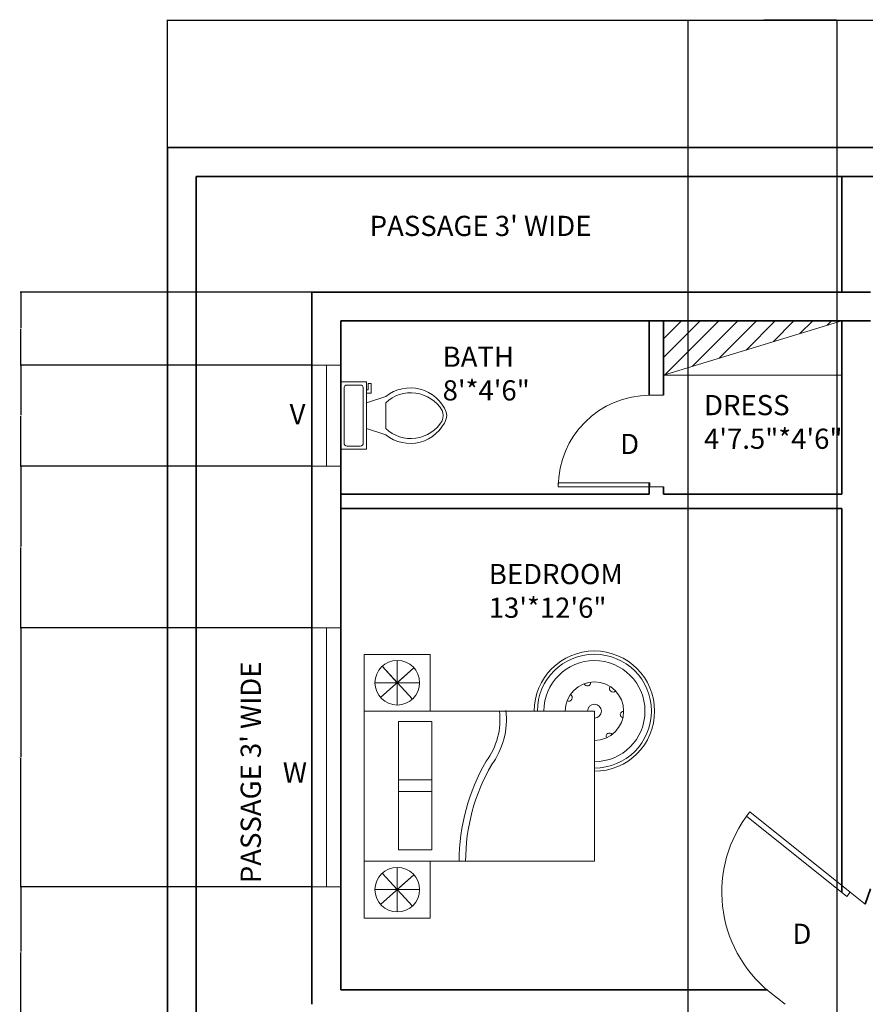
# Model space of a CAD drawing. Units: inches. Extents: x 2284 to 2815, y 1123 to 1948.
# Tile 5 of 6: x 2285 to 2548, y 1641 to 1948. Entities that reach past the tile are written whole.
import ezdxf

# ---------------------------------------------------------------- set-up
doc = ezdxf.new("R2010")
doc.units = ezdxf.units.IN
for name, color, linetype, lineweight in [('A-ANNO-DIMS', 2, 'Continuous', 18), ('A-AREA-IDEN', 30, 'Continuous', 18), ('A-CASE-PATT', 217, 'Continuous', 13), ('A-FLOR-CASE', 8, 'Continuous', 18), ('A-FLOR-FIXT', 9, 'Continuous', 18), ('A-WALL-PATT', 140, 'Continuous', 13), ('C-SITE-WALL', 7, 'Continuous', 35), ('DOOR', 190, 'Continuous', 18), ('FUR', 10, 'Continuous', 18), ('TEXT', 30, 'Continuous', 18), ('WALL', 7, 'Continuous', 35), ('WIND', 210, 'Continuous', 18)]:
    doc.layers.add(name, color=color, linetype=linetype, lineweight=lineweight)
doc.styles.get("Standard").update_dxf_attribs({"font": 'arial.ttf'})
doc.dimstyles.get("Standard").update_dxf_attribs({"dimtxt": 0.18, "dimasz": 0.18, "dimexe": 0.18, "dimexo": 0.0625, "dimgap": 0.09, "dimtad": 0, "dimtih": 1, "dimtoh": 1, "dimdec": 4, "dimzin": 0, "dimdsep": 46, "dimtxsty": 'Standard', "dimcen": 0.09, "dimadec": 0, "dimazin": 0, "dimtfac": 1, "dimtdec": 4, "dimtofl": 0, "dimtmove": 0, "dimatfit": 3, "dimfxl": 1, "dimtolj": 1, "dimtzin": 0, "dimarcsym": 0})

# ---------------------------------------------------------------- blocks, each defined once
blk = doc.blocks.new('*U2')
for p, q in [((0, 0), (0, -6)), ((40, 0), (40, -6))]:
    blk.add_line(p, q)
blk.add_lwpolyline([(0, 0), (0, 40), (1.75, 40), (1.75, 0)], close=True)
blk.add_arc((0, 0), 40, 0, 90)
blk = doc.blocks.new('*U4')
for p, q in [((9.5, -6), (9.5, -2)), ((-10, -8.5), (-8, -8.5)), ((-10, -9.5), (-10, -8.5)), ((-8, -8.5), (-8, -8)), ((-7, -8), (-7, -9.5)), ((-4, -8), (-6, -14)), ((4, -8), (6, -14)), ((-7, -9.5), (-10, -9.5)), ((4, -14), (-4, -14))]:
    blk.add_line(p, q)
blk.add_lwpolyline([(10.5, -8), (10.5, 0), (-10.5, 0), (-10.5, -8)], close=True)
for points in [[(-9.5, -2), (-9.5, -6)], [(8.5, -1), (-8.5, -1)], [(-8.5, -7), (8.5, -7)]]:
    blk.add_lwpolyline(points)
for centre, radius, start, end in [((-8.62, -1.88), 0.884, 81.8699, 188.1301), ((8.62, -1.88), 0.884, 351.8699, 98.1301), ((-8.62, -6.12), 0.884, 171.8699, 278.1301), ((8.62, -6.12), 0.884, 261.8699, 8.1301), ((3.52, -21.58), 12.17, 141.4691, 247.9714), ((4.2, -21.82), 11.33, 136.3677, 238.9468), ((-3.52, -21.58), 12.17, 292.0284, 38.5307), ((-4.2, -21.82), 11.33, 301.053, 43.6321), ((0, -27.88), 4, 245.7318, 294.2682), ((0, -29), 4, 254.8605, 285.1395)]:
    blk.add_arc(centre, radius, start, end)
blk = doc.blocks.new('BED-DOUBLE-WITH-RUG')
for points in [[(0, 0), (71.68, 0), (71.68, 46.8), (0, 46.8)], [(10.67, 21.75), (21.03, 21.75), (21.03, 43.61), (10.67, 43.61)], [(10.67, 3.58), (21.03, 3.58), (21.03, 25.43), (10.67, 25.43)]]:
    blk.add_lwpolyline(points, close=True)
for centre, radius, start, end in [((71.68, 46.8), 18.75, 270, 180), ((71.68, 46.8), 17.75, 270, 180), ((71.68, 46.8), 15.75, 270, 180), ((71.68, 46.8), 9.1, 270, 180), ((69.48, 55.63), 1, 197.1257, 10.8048), ((77.45, 53.83), 1.1, 144.137, 317.2027), ((63.62, 51.01), 1.12, 245.9164, 58.891), ((20.54, 44.16), 21.72, 323.3068, 6.9612), ((20.54, 44.16), 23.72, 323.3068, 6.9612), ((71.68, 46.8), 2.16, 270, 180), ((80.72, 45.75), 0.986, 86.4879, 260.2794), ((76.34, 38.98), 1, 33.9622, 207.6652), ((91.6, 0), 62.04, 149.8305, 180), ((91.6, 0), 60.04, 149.8305, 180)]:
    blk.add_arc(centre, radius, start, end)
blk = doc.blocks.new('NIGHTSTAND-LAMP')
for p, q in [((10.28, 1.89), (10.28, 15.8)), ((15.48, 13.46), (5.08, 4.23)), ((10.28, 8.85), (5.59, 13.98)), ((5.59, 13.98), (14.97, 3.71)), ((10.28, 8.85), (15.48, 13.46)), ((3.33, 8.85), (17.23, 8.85))]:
    blk.add_line(p, q)
blk.add_lwpolyline([(0, 0), (20.56, 0), (20.56, 17.69), (0, 17.69)], close=True)
blk.add_circle((10.28, 8.85), 6.95)
blk = doc.blocks.new('*D20')
at = {"layer": 'A-ANNO-DIMS', "color": 0, "lineweight": -2, "transparency": 16777216}
for p, q in [((2330.55, 1908.47), (2330.55, 1948.28)), ((2330.73, 1948.1), (2552.26, 1948.1)), ((2774.37, 1948.1), (2552.85, 1948.1)), ((2774.55, 1908.47), (2774.55, 1948.28))]:
    blk.add_line(p, q, dxfattribs=at)
at = {"layer": 'A-ANNO-DIMS', "color": 0, "transparency": 16777216}
for points in [[(2330.73, 1948.13), (2330.73, 1948.07), (2330.55, 1948.1)], [(2774.37, 1948.13), (2774.37, 1948.07), (2774.55, 1948.1)]]:
    blk.add_solid(points, dxfattribs=at)
at = {"layer": 'Defpoints', "color": 0, "transparency": 16777216}
for p in [(2774.55, 1948.1), (2330.55, 1908.4), (2774.55, 1908.4)]:
    blk.add_point(p, dxfattribs=at)
at = {"layer": 'A-ANNO-DIMS', "color": 0, "transparency": 16777216, "insert": (2552.55, 1948.1), "char_height": 0.18, "attachment_point": 5}
blk.add_mtext('\\A1;444', dxfattribs=at)
blk = doc.blocks.new('*D32')
at = {"layer": 'A-ANNO-DIMS', "color": 0, "lineweight": -2, "transparency": 16777216}
for p, q in [((2375.49, 1678.06), (2284.67, 1678.06)), ((2284.85, 1677.88), (2284.85, 1657.9)), ((2284.85, 1637.55), (2284.85, 1657.53)), ((2375.49, 1637.37), (2284.67, 1637.37))]:
    blk.add_line(p, q, dxfattribs=at)
at = {"layer": 'A-ANNO-DIMS', "color": 0, "transparency": 16777216}
for points in [[(2284.82, 1677.88), (2284.88, 1677.88), (2284.85, 1678.06)], [(2284.82, 1637.55), (2284.88, 1637.55), (2284.85, 1637.37)]]:
    blk.add_solid(points, dxfattribs=at)
at = {"layer": 'Defpoints', "color": 0, "transparency": 16777216}
for p in [(2284.85, 1678.06), (2375.55, 1678.06), (2375.55, 1637.37)]:
    blk.add_point(p, dxfattribs=at)
at = {"layer": 'A-ANNO-DIMS', "color": 0, "transparency": 16777216, "insert": (2284.85, 1657.71), "char_height": 0.18, "attachment_point": 5}
blk.add_mtext('\\A1;40.69', dxfattribs=at)
blk = doc.blocks.new('*D33')
at = {"layer": 'A-ANNO-DIMS', "color": 0, "lineweight": -2, "transparency": 16777216}
for p, q in [((2375.49, 1758.74), (2284.67, 1758.74)), ((2284.85, 1758.56), (2284.85, 1718.58)), ((2284.85, 1678.24), (2284.85, 1718.22)), ((2375.49, 1678.06), (2284.67, 1678.06))]:
    blk.add_line(p, q, dxfattribs=at)
at = {"layer": 'A-ANNO-DIMS', "color": 0, "transparency": 16777216}
for points in [[(2284.82, 1758.56), (2284.88, 1758.56), (2284.85, 1758.74)], [(2284.82, 1678.24), (2284.88, 1678.24), (2284.85, 1678.06)]]:
    blk.add_solid(points, dxfattribs=at)
at = {"layer": 'Defpoints', "color": 0, "transparency": 16777216}
for p in [(2284.85, 1758.74), (2375.55, 1758.74), (2375.55, 1678.06)]:
    blk.add_point(p, dxfattribs=at)
at = {"layer": 'A-ANNO-DIMS', "color": 0, "transparency": 16777216, "insert": (2284.85, 1718.4), "char_height": 0.18, "attachment_point": 5}
blk.add_mtext('\\A1;80.68', dxfattribs=at)
blk = doc.blocks.new('*D34')
at = {"layer": 'A-ANNO-DIMS', "color": 0, "lineweight": -2, "transparency": 16777216}
for p, q in [((2375.49, 1809.15), (2284.67, 1809.15)), ((2284.85, 1808.97), (2284.85, 1784.13)), ((2284.85, 1758.92), (2284.85, 1783.77)), ((2375.49, 1758.74), (2284.67, 1758.74))]:
    blk.add_line(p, q, dxfattribs=at)
at = {"layer": 'A-ANNO-DIMS', "color": 0, "transparency": 16777216}
for points in [[(2284.82, 1808.97), (2284.88, 1808.97), (2284.85, 1809.15)], [(2284.82, 1758.92), (2284.88, 1758.92), (2284.85, 1758.74)]]:
    blk.add_solid(points, dxfattribs=at)
at = {"layer": 'Defpoints', "color": 0, "transparency": 16777216}
for p in [(2284.85, 1809.15), (2375.55, 1809.15), (2375.55, 1758.74)]:
    blk.add_point(p, dxfattribs=at)
at = {"layer": 'A-ANNO-DIMS', "color": 0, "transparency": 16777216, "insert": (2284.85, 1783.95), "char_height": 0.18, "attachment_point": 5}
blk.add_mtext('\\A1;50.41', dxfattribs=at)
blk = doc.blocks.new('*D35')
at = {"layer": 'A-ANNO-DIMS', "color": 0, "lineweight": -2, "transparency": 16777216}
for p, q in [((2375.49, 1840.6), (2284.67, 1840.6)), ((2284.85, 1840.42), (2284.85, 1825.06)), ((2284.85, 1809.33), (2284.85, 1824.7)), ((2375.49, 1809.15), (2284.67, 1809.15))]:
    blk.add_line(p, q, dxfattribs=at)
at = {"layer": 'A-ANNO-DIMS', "color": 0, "transparency": 16777216}
for points in [[(2284.82, 1840.42), (2284.88, 1840.42), (2284.85, 1840.6)], [(2284.82, 1809.33), (2284.88, 1809.33), (2284.85, 1809.15)]]:
    blk.add_solid(points, dxfattribs=at)
at = {"layer": 'Defpoints', "color": 0, "transparency": 16777216}
for p in [(2284.85, 1840.6), (2375.55, 1840.6), (2375.55, 1809.15)]:
    blk.add_point(p, dxfattribs=at)
at = {"layer": 'A-ANNO-DIMS', "color": 0, "transparency": 16777216, "insert": (2284.85, 1824.88), "char_height": 0.18, "attachment_point": 5}
blk.add_mtext('\\A1;31.45', dxfattribs=at)
blk = doc.blocks.new('*D36')
at = {"layer": 'A-ANNO-DIMS', "color": 0, "lineweight": -2, "transparency": 16777216}
for p, q in [((2375.49, 1863.4), (2284.67, 1863.4)), ((2284.85, 1863.22), (2284.85, 1852.18)), ((2284.85, 1840.78), (2284.85, 1851.82)), ((2375.49, 1840.6), (2284.67, 1840.6))]:
    blk.add_line(p, q, dxfattribs=at)
at = {"layer": 'A-ANNO-DIMS', "color": 0, "transparency": 16777216}
for points in [[(2284.82, 1863.22), (2284.88, 1863.22), (2284.85, 1863.4)], [(2284.82, 1840.78), (2284.88, 1840.78), (2284.85, 1840.6)]]:
    blk.add_solid(points, dxfattribs=at)
at = {"layer": 'Defpoints', "color": 0, "transparency": 16777216}
for p in [(2284.85, 1863.4), (2375.55, 1863.4), (2375.55, 1840.6)]:
    blk.add_point(p, dxfattribs=at)
at = {"layer": 'A-ANNO-DIMS', "color": 0, "transparency": 16777216, "insert": (2284.85, 1852), "char_height": 0.18, "attachment_point": 5}
blk.add_mtext('\\A1;22.8', dxfattribs=at)
blk = doc.blocks.new('*D46')
at = {"layer": 'A-ANNO-DIMS', "color": 0, "lineweight": -2, "transparency": 16777216}
for p, q in [((2492.72, 1419.47), (2492.72, 1948.28)), ((2492.9, 1948.1), (2515.54, 1948.1)), ((2538.95, 1948.1), (2516.3, 1948.1)), ((2539.13, 1419.47), (2539.13, 1948.28))]:
    blk.add_line(p, q, dxfattribs=at)
at = {"layer": 'A-ANNO-DIMS', "color": 0, "transparency": 16777216}
for points in [[(2492.9, 1948.13), (2492.9, 1948.07), (2492.72, 1948.1)], [(2538.95, 1948.13), (2538.95, 1948.07), (2539.13, 1948.1)]]:
    blk.add_solid(points, dxfattribs=at)
at = {"layer": 'Defpoints', "color": 0, "transparency": 16777216}
for p in [(2539.13, 1948.1), (2492.72, 1419.4), (2539.13, 1419.4)]:
    blk.add_point(p, dxfattribs=at)
at = {"layer": 'A-ANNO-DIMS', "color": 0, "transparency": 16777216, "insert": (2515.92, 1948.1), "char_height": 0.18, "attachment_point": 5}
blk.add_mtext('\\A1;46.41', dxfattribs=at)

msp = doc.modelspace()

# ---------------------------------------------------------------- hatches: boundary and pattern name
at = {"layer": 'A-CASE-PATT'}
h = msp.add_hatch(dxfattribs=at)
h.set_pattern_fill('ANSI31', color=256, scale=1.3)
h.paths.add_polyline_path([(2765.554, 1774.904), (2744.1119, 1774.904), (2765.554, 1686.404)])
h.paths.add_polyline_path([(2540.554, 1854.404), (2485.054, 1854.404), (2485.054, 1837.4988)])
at = {"layer": 'A-WALL-PATT'}
h = msp.add_hatch(dxfattribs=at)
h.set_pattern_fill('AR-SAND', color=256, scale=8.5)
h.paths.add_polyline_path([(2339.554, 1899.404), (2375.554, 1899.404), (2765.554, 1899.404), (2765.554, 1185.404), (2549.3222, 1185.404), (2549.3222, 1176.404), (2774.554, 1176.404), (2774.554, 1908.404), (2330.554, 1908.404), (2330.554, 1176.404), (2349.4276, 1176.404), (2349.4276, 1185.404), (2339.554, 1185.404)])
h.paths.add_polyline_path([(2710.054, 1899.404), (2701.054, 1899.404), (2701.054, 1889.8374), (2710.054, 1889.8374)], flags=17)
h = msp.add_hatch(dxfattribs=at)
h.set_pattern_fill('AR-SAND', color=256, scale=8.5)
h.paths.add_polyline_path([(2549.554, 1863.404), (2375.554, 1863.404), (2375.554, 1840.6021), (2384.554, 1840.6021), (2384.554, 1854.404), (2480.554, 1854.404), (2549.554, 1854.404)])
h.paths.add_polyline_path([(2384.554, 1795.904), (2384.554, 1809.1528), (2375.554, 1809.1528), (2375.554, 1758.7416), (2384.554, 1758.7416)])
h.paths.add_polyline_path([(2549.554, 1836.404), (2549.554, 1854.404), (2540.554, 1854.404), (2540.554, 1800.404), (2485.054, 1800.404), (2485.054, 1802.7347), (2480.554, 1802.7347), (2480.554, 1800.404), (2384.554, 1800.404), (2384.554, 1795.904), (2485.054, 1795.904), (2540.554, 1795.904), (2540.554, 1678.5102), (2543.2164, 1676.3784), (2547.9, 1672.6283), (2549.554, 1677.404), (2549.554, 1795.904)])
h.paths.add_polyline_path([(2452.31, 1803.9815), (2480.7795, 1803.9815), (2480.7795, 1802.7347), (2452.2828, 1802.7347), (2452.2828, 1803.9815), (2452.31, 1803.9815, -0.39915744), (2480.554, 1831.2306), (2480.554, 1854.404), (2540.554, 1854.404), (2485.054, 1837.4988), (2485.054, 1831.2315), (2480.7795, 1831.2315, 0.40145271)], flags=17)
h.paths.add_polyline_path([(2583.189, 1845.404), (2549.554, 1845.404), (2549.554, 1836.404), (2583.189, 1836.404)])
h.paths.add_polyline_path([(2710.054, 1858.3882), (2701.054, 1858.3882), (2701.054, 1845.404), (2671.4007, 1845.404), (2671.4007, 1836.404), (2710.054, 1836.404)])
h.paths.add_polyline_path([(2710.054, 1836.404), (2705.554, 1836.404), (2705.554, 1774.904), (2710.054, 1774.904), (2710.054, 1779.404)])
h.paths.add_polyline_path([(2765.554, 1779.404), (2737.9116, 1779.404, -0.00645116), (2737.9201, 1778.7436), (2737.9201, 1774.904), (2765.554, 1774.904)])
h.paths.add_polyline_path([(2712.3231, 1778.7436), (2712.3231, 1779.404), (2710.054, 1779.404), (2710.054, 1774.904), (2712.3231, 1774.904)])
h.paths.add_polyline_path([(2710.054, 1774.904), (2705.554, 1774.904), (2705.554, 1769.4647), (2710.054, 1769.4647)])
h.paths.add_polyline_path([(2710.054, 1702.7233), (2705.554, 1702.7233), (2705.554, 1686.404), (2592.0733, 1686.404, -0.01876983), (2592.186, 1683.404), (2592.186, 1677.404), (2705.554, 1677.404), (2765.554, 1677.404), (2765.554, 1686.404), (2710.054, 1686.404)])
h.paths.add_polyline_path([(2384.554, 1641.404), (2375.554, 1641.404), (2375.554, 1637.3708), (2381.554, 1637.3708), (2384.554, 1637.3708)])
h.paths.add_polyline_path([(2384.554, 1678.0573), (2375.554, 1678.0573), (2375.554, 1641.404), (2384.554, 1641.404), (2522.8991, 1641.404), (2518.2155, 1645.1541, -0.00736412), (2517.3067, 1645.904), (2384.554, 1645.904)])
h.paths.add_polyline_path([(2384.554, 1597.4834, -0.01876983), (2381.554, 1597.3708), (2375.554, 1597.3708), (2375.554, 1591.564), (2384.554, 1591.564)])
h.paths.add_polyline_path([(2384.554, 1533.404), (2384.554, 1538.4896), (2375.554, 1538.4896), (2375.554, 1524.404), (2384.554, 1524.404)])
h.paths.add_polyline_path([(2506.054, 1533.404), (2506.054, 1598.7748), (2500.054, 1598.7748, -0.01876983), (2497.054, 1598.8874), (2497.054, 1533.404), (2384.554, 1533.404), (2384.554, 1524.404), (2497.054, 1524.404), (2506.054, 1524.404)])
h.paths.add_polyline_path([(2473.054, 1446.985), (2468.9674, 1446.985, -0.00379375), (2468.554, 1446.9881), (2468.554, 1428.404), (2473.054, 1428.404)])
h.paths.add_polyline_path([(2384.554, 1524.404), (2375.554, 1524.404), (2375.554, 1468.4232), (2384.554, 1468.4232)])
h.paths.add_polyline_path([(2473.054, 1480.904), (2384.554, 1480.904), (2384.554, 1476.404), (2468.554, 1476.404), (2468.554, 1474.2289), (2468.9674, 1474.2289), (2473.054, 1474.2289)])
h.paths.add_polyline_path([(2555.554, 1428.404), (2546.554, 1428.404), (2539.1317, 1428.404), (2539.1317, 1422.885), (2539.1317, 1419.404), (2546.554, 1419.404), (2555.554, 1419.404)])
h.paths.add_polyline_path([(2564.554, 1368.404), (2564.554, 1370.9838), (2561.554, 1370.9838), (2555.554, 1370.9838), (2555.554, 1359.404), (2564.554, 1359.404)])
h.paths.add_polyline_path([(2623.1768, 1368.404), (2564.554, 1368.404), (2564.554, 1359.404), (2623.1768, 1359.404)])
h.paths.add_polyline_path([(2492.7181, 1422.885), (2492.7181, 1428.404), (2384.554, 1428.404), (2384.554, 1440.6426), (2375.554, 1440.6426), (2375.554, 1419.404), (2492.7181, 1419.404)])
h.paths.add_polyline_path([(2765.554, 1368.404), (2710.406, 1368.404), (2710.406, 1359.404), (2765.554, 1359.404)])
h.paths.add_polyline_path([(2765.554, 1533.404), (2732.876, 1533.404), (2732.876, 1524.404), (2765.554, 1524.404)])
h.paths.add_polyline_path([(2624.1792, 1533.404), (2599.5288, 1533.404), (2590.3672, 1524.404), (2564.554, 1499.046), (2555.554, 1490.2048), (2555.554, 1410.9838), (2561.554, 1410.9838, -0.01876983), (2564.554, 1410.8712), (2564.554, 1486.4298), (2603.2099, 1524.404), (2624.1792, 1524.404)])
h.paths.add_polyline_path([(2555.554, 1490.2048), (2556.4043, 1491.0401), (2549.047, 1496.8538), (2545.7227, 1492.1958), (2543.8126, 1489.5193), (2555.554, 1480.2413)])
h.paths.add_polyline_path([(2514.6892, 1524.0031), (2506.054, 1530.8266), (2506.054, 1524.404), (2499.6656, 1524.404), (2500.474, 1523.7652), (2509.4548, 1516.6686), (2511.3649, 1519.3451)])
h.paths.add_polyline_path([(2365.9834, 1447.3726), (2374.9891, 1447.3726), (2374.9891, 1460.3342), (2365.9834, 1460.3342)], flags=9)
h.paths.add_polyline_path([(2366.9945, 1818.7713), (2376.0002, 1818.7713), (2376.0002, 1831.7328), (2366.9945, 1831.7328)], flags=9)
h.paths.add_polyline_path([(2363.2989, 1558.2059), (2374.7373, 1558.2059), (2374.7373, 1571.1674), (2363.2989, 1571.1674)], flags=9)
h.paths.add_polyline_path([(2364.8137, 1707.1012), (2376.2521, 1707.1012), (2376.2521, 1720.0627), (2364.8137, 1720.0627)], flags=9)
h.paths.add_polyline_path([(2460.3189, 1455.9932), (2469.8094, 1455.9932), (2469.8094, 1468.9547), (2460.3189, 1468.9547)], flags=9)
h.paths.add_polyline_path([(2558.6325, 1386.2225), (2568.1231, 1386.2225), (2568.1231, 1399.184), (2558.6325, 1399.184)], flags=9)
h.paths.add_polyline_path([(2378.5629, 1611.6816), (2388.0534, 1611.6816), (2388.0534, 1624.6431), (2378.5629, 1624.6431)], flags=9)
h.paths.add_polyline_path([(2490.2277, 1613.2326), (2499.7182, 1613.2326), (2499.7182, 1626.1941), (2490.2277, 1626.1941)], flags=9)
h.paths.add_polyline_path([(2522.9652, 1656.7942), (2532.4557, 1656.7942), (2532.4557, 1669.7557), (2522.9652, 1669.7557)], flags=9)
h.paths.add_polyline_path([(2567.5462, 1677.3031), (2577.0367, 1677.3031), (2577.0367, 1690.2646), (2567.5462, 1690.2646)], flags=9)
h.paths.add_polyline_path([(2363.196, 1676.9136), (2363.196, 1756.4461), (2350.2345, 1756.4461), (2350.2345, 1676.9136)], flags=9)
h.paths.add_polyline_path([(2515.5569, 1505.5998), (2535.7182, 1488.4964), (2539.8301, 1493.3434), (2519.6687, 1510.4468)], flags=9)
h.paths.add_polyline_path([(2503.6006, 1414.6146), (2530.0393, 1414.6146), (2530.0393, 1420.9707), (2503.6006, 1420.9707)], flags=9)
h.paths.add_polyline_path([(2391.2946, 1877.326), (2470.827, 1877.326), (2470.827, 1890.2876), (2391.2946, 1890.2876)], flags=9)
h.paths.add_polyline_path([(2580.3233, 1794.4386), (2629.1831, 1794.4386), (2629.1831, 1817.9089), (2580.3233, 1817.9089)], flags=9)
h.paths.add_polyline_path([(2585.6043, 1595.2228), (2648.3653, 1595.2228), (2648.3653, 1618.6931), (2585.6043, 1618.6931)], flags=9)
h.paths.add_polyline_path([(2591.9981, 1445.0189), (2637.889, 1445.0189), (2637.889, 1468.4892), (2591.9981, 1468.4892)], flags=9)
h.paths.add_polyline_path([(2459.0727, 1376.5795), (2515.4624, 1376.5795), (2515.4624, 1400.0498), (2459.0727, 1400.0498)], flags=9)
h.paths.add_polyline_path([(2481.8769, 1451.6363), (2543.2049, 1451.6363), (2543.2049, 1475.1066), (2481.8769, 1475.1066)], flags=9)
h.paths.add_polyline_path([(2470.0329, 1495.943), (2485.3842, 1495.943), (2485.3842, 1508.9045), (2470.0329, 1508.9045)], flags=9)
h.paths.add_polyline_path([(2419.5143, 1438.0898), (2446.0938, 1438.0898), (2446.0938, 1461.5344), (2419.5143, 1461.5344)], flags=9)
h.paths.add_polyline_path([(2425.6893, 1570.7133), (2467.4012, 1570.7133), (2467.4012, 1594.1836), (2425.6893, 1594.1836)], flags=25)
h.paths.add_polyline_path([(2428.101, 1758.2973), (2476.9609, 1758.2973), (2476.9609, 1781.7676), (2428.101, 1781.7676)], flags=25)

# ---------------------------------------------------------------- linework, layer by layer
at = {"layer": 'A-FLOR-CASE'}
for q in [(2540.554, 1854.404), (2540.554, 1837.4988)]:
    msp.add_line((2485.054, 1837.4988), q, dxfattribs=at)
at = {"layer": 'C-SITE-WALL'}
for p, q in [((2330.554, 1908.404), (2774.554, 1908.404)), ((2330.554, 1176.404), (2330.554, 1908.404)), ((2339.554, 1185.404), (2339.554, 1899.404)), ((2339.554, 1899.404), (2765.554, 1899.404)), ((2339.554, 1899.404), (2375.554, 1899.404)), ((2339.554, 1899.404), (2375.554, 1899.404)), ((2339.554, 1899.404), (2339.554, 1863.404)), ((2540.554, 1899.404), (2701.054, 1899.404))]:
    msp.add_line(p, q, dxfattribs=at)
at = {"layer": 'WALL'}
for p, q in [((2540.554, 1863.404), (2540.554, 1899.404)), ((2375.554, 1863.404), (2375.554, 1840.6021)), ((2375.554, 1863.404), (2549.554, 1863.404)), ((2384.554, 1854.404), (2549.554, 1854.404)), ((2384.554, 1854.404), (2384.554, 1714.7105)), ((2384.554, 1854.404), (2384.554, 1840.6021)), ((2384.554, 1854.404), (2480.554, 1854.404)), ((2480.554, 1854.404), (2480.554, 1831.2306)), ((2485.054, 1854.404), (2485.054, 1831.2315)), ((2485.054, 1854.404), (2540.554, 1854.404)), ((2540.554, 1854.404), (2540.554, 1800.404)), ((2375.554, 1840.6021), (2375.554, 1714.7105)), ((2480.554, 1803.9815), (2480.554, 1800.404)), ((2485.054, 1802.7347), (2485.054, 1800.404)), ((2480.554, 1800.404), (2384.554, 1800.404)), ((2540.554, 1800.404), (2485.054, 1800.404)), ((2485.054, 1795.904), (2384.554, 1795.904)), ((2384.554, 1795.904), (2384.554, 1645.904)), ((2540.554, 1795.904), (2485.054, 1795.904)), ((2540.554, 1676.2683), (2540.554, 1795.904)), ((2375.554, 1714.7105), (2375.554, 1641.404)), ((2547.9, 1672.6283), (2549.554, 1677.404)), ((2384.554, 1645.904), (2517.4792, 1645.904))]:
    msp.add_line(p, q, dxfattribs=at)
at = {"layer": 'WIND'}
for p, q in [((2380.054, 1809.1528), (2380.054, 1840.6021)), ((2380.054, 1678.0573), (2380.054, 1758.7416))]:
    msp.add_line(p, q, dxfattribs=at)
for points in [[(2384.554, 1840.6021), (2375.554, 1840.6021), (2375.554, 1809.1528), (2384.554, 1809.1528)], [(2375.554, 1678.0573), (2384.554, 1678.0573), (2384.554, 1758.7416), (2375.554, 1758.7416)]]:
    msp.add_lwpolyline(points, close=True, dxfattribs=at)

# ---------------------------------------------------------------- block references
at = {"layer": 'A-FLOR-FIXT', "xscale": -1, "rotation": 90}
msp.add_blockref('*U4', (2384.554, 1824.8774), dxfattribs=at)
at = {"layer": 'DOOR', "xscale": 0.712417595267903, "yscale": 0.712417595267903, "zscale": 0.712417595267903, "rotation": 90}
msp.add_blockref('*U2', (2480.7795, 1802.7347), dxfattribs=at)
at = {"layer": 'DOOR', "xscale": -1, "rotation": 51.31614925736204}
msp.add_blockref('*U2', (2543.2164, 1676.3784), dxfattribs=at)
at = {"layer": 'FUR'}
for name, p in [('BED-DOUBLE-WITH-RUG', (2391.861, 1685.976)), ('NIGHTSTAND-LAMP', (2391.861, 1732.771)), ('NIGHTSTAND-LAMP', (2391.861, 1668.2856))]:
    msp.add_blockref(name, p, dxfattribs=at)

# ---------------------------------------------------------------- texts
at = {"layer": 'A-AREA-IDEN', "attachment_point": 1}
for s, insert, char_height in [("PASSAGE 3' WIDE", (2393.5449, 1887.1577), 6.289829), ('BATH\\P8\'*4\'6"', (2416.265, 1846.3795), 6.28983), ('DRESS\\P4\'7.5"*4\'6"', (2497.6817, 1831.3039), 6.289829), ('BEDROOM\\P13\'*12\'6"', (2430.6302, 1778.642), 6.28983)]:
    msp.add_mtext_dynamic_manual_height_columns(s, width=114.078767, gutter_width=31.4491, heights=[0], dxfattribs=dict(at, insert=insert, char_height=char_height))
at = {"layer": 'A-AREA-IDEN', "insert": (2353.3644, 1679.164), "char_height": 6.289829, "attachment_point": 1, "rotation": 90}
msp.add_mtext_dynamic_manual_height_columns("PASSAGE 3' WIDE", width=114.078767, gutter_width=31.4491, heights=[0], dxfattribs=at)
at = {"layer": 'TEXT', "char_height": 6.2898, "attachment_point": 1}
for s, insert in [('V', (2368.6056, 1828.4957)), ('D', (2471.5598, 1819.1838)), ('W', (2366.4934, 1716.8255)), ('D', (2525.2155, 1666.5186))]:
    msp.add_mtext_dynamic_manual_height_columns(s, width=114.078767, gutter_width=31.4491, heights=[0], dxfattribs=dict(at, insert=insert))

# ---------------------------------------------------------------- dimensions: what is measured, and where the dimension line sits
at = {"layer": 'A-ANNO-DIMS'}
for base, p1, p2, override, picture, middle in [((2774.554, 1948.104), (2330.554, 1908.404), (2774.554, 1908.404), {"dimdec": 0, "dimlfac": 1, "dimrnd": 0, "dimzin": 0, "dimdsep": 46, "dimlunit": 2}, '*D20', (2552.554, 1948.104)), ((2539.1317, 1948.104), (2492.7181, 1419.404), (2539.1317, 1419.404), {"dimdec": 2, "dimlfac": 1, "dimrnd": 0, "dimzin": 0, "dimdsep": 46, "dimlunit": 2}, '*D46', (2515.9249, 1948.104))]:
    dim = msp.add_linear_dim(base=base, p1=p1, p2=p2, dimstyle='Standard', override=override, dxfattribs=at)
    dim.commit()
    dim.dimension.update_dxf_attribs({"geometry": picture, "text_midpoint": middle})
for base, p1, p2, override, picture, middle in [((2284.854, 1863.404), (2375.554, 1840.6021), (2375.554, 1863.404), {"dimdec": 1, "dimlfac": 1, "dimrnd": 0, "dimzin": 0, "dimdsep": 46, "dimlunit": 2}, '*D36', (2284.854, 1852.003)), ((2284.854, 1840.6021), (2375.554, 1809.1528), (2375.554, 1840.6021), {"dimdec": 2, "dimlfac": 1, "dimrnd": 0, "dimzin": 0, "dimdsep": 46, "dimlunit": 2}, '*D35', (2284.854, 1824.8774)), ((2284.854, 1809.1528), (2375.554, 1758.7416), (2375.554, 1809.1528), {"dimdec": 2, "dimlfac": 1, "dimrnd": 0, "dimzin": 0, "dimdsep": 46, "dimlunit": 2}, '*D34', (2284.854, 1783.9472)), ((2284.854, 1758.7416), (2375.554, 1678.0573), (2375.554, 1758.7416), {"dimdec": 2, "dimlfac": 1, "dimrnd": 0, "dimzin": 0, "dimdsep": 46, "dimlunit": 2}, '*D33', (2284.854, 1718.3994)), ((2284.854, 1678.0573), (2375.554, 1637.3708), (2375.554, 1678.0573), {"dimdec": 2, "dimlfac": 1, "dimrnd": 0, "dimzin": 0, "dimdsep": 46, "dimlunit": 2}, '*D32', (2284.854, 1657.714))]:
    dim = msp.add_linear_dim(base=base, p1=p1, p2=p2, angle=90, dimstyle='Standard', override=override, dxfattribs=at)
    dim.commit()
    dim.dimension.update_dxf_attribs({"geometry": picture, "text_midpoint": middle})

doc.saveas('drawing.dxf')
